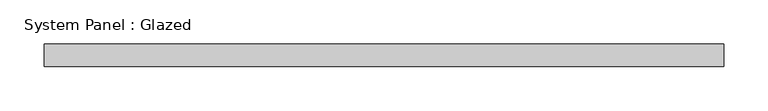
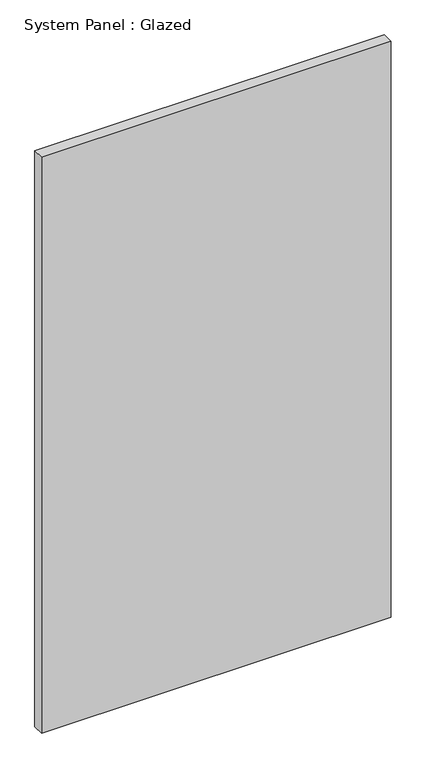
"""IFC4 building model written with IfcOpenShell, lengths in millimetres: plate geometry, System Panel : Glazed."""

from ifc_helpers import new_model, si_unit, origin, origin_with_axes, place, context, project, spatial, polyline, outline, extrude, source, transform, mapped, element, save


def system_panel_glazed_78f80fad(model_context):
    return source(origin(), model_context, "Body", "SweptSolid", [
        extrude(outline(polyline([(382.2267437, 24.5), (-382.2267437, 24.5), (-382.2267437, 49.5), (382.2267437, 49.5), (382.2267437, 24.5)])), origin_with_axes(), (0.0, 0.0, 1.0), 1330.8429687),
    ])


if __name__ == "__main__":
    model = new_model("IFC4")
    model_context = context("Model", 3, world=origin())
    ifc_project = project(units=[si_unit("LENGTHUNIT", "METRE", prefix="MILLI")], contexts=[model_context])
    site = spatial("IfcSite", under=ifc_project)
    building = spatial("IfcBuilding", under=site)
    placement = place(None, origin())
    system_panel_glazed_shape = system_panel_glazed_78f80fad(model_context)
    element("IfcPlate", 1, ObjectType="System Panel : Glazed", at=placement, inside=building, context=model_context, shape_type="MappedRepresentation", body=[
        mapped(system_panel_glazed_shape, transform((0.0, 0.0, 0.0), x_axis=(1.0, 0.0, 0.0), y_axis=(0.0, 1.0, 0.0), z_axis=(0.0, 0.0, 1.0))),
    ])
    save(model, "model.ifc")

# Revit data of these elements
# Type "System Panel : Glazed"
#   Keynote = "H11"
#   Construction Type Id = "GSP4R"
#   Analytic Construction = "1/8 in Pilkington single glazing"
#   Visual Light Transmittance = 0.9
#   Solar Heat Gain Coefficient = 0.86
#   Heat Transfer Coefficient (U) = 6.7069 W/(m²·K)
#   Define Thermal Properties by = 1
# Element 1 (IfcPlate, "System Panel : Glazed")
#   Materials on its faces: "Glass"
# Materials
#   "Glass": class "Glass", colour RGB 0 128 192, transparency 0.9, Description = "Soda Lime Glass", Cost = 0
